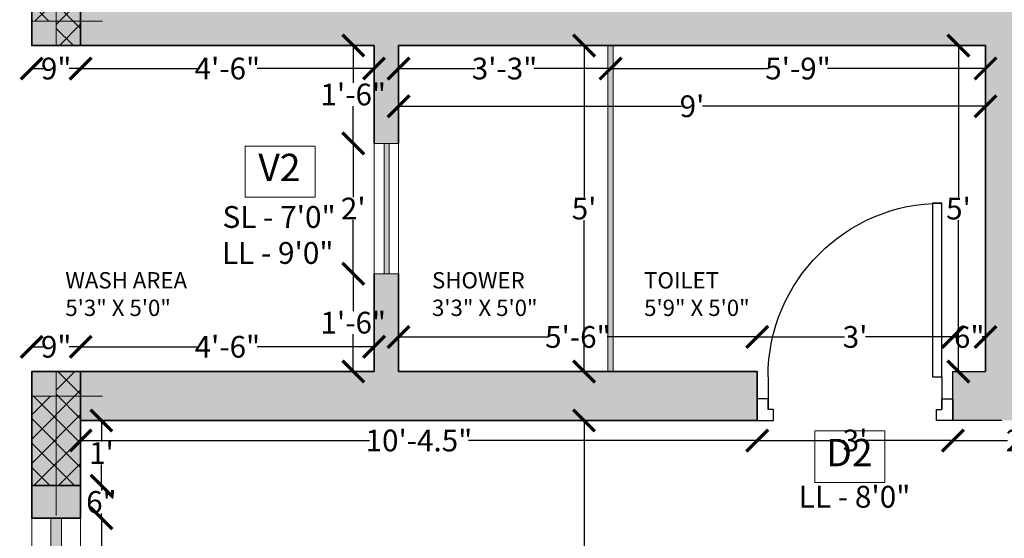
# Model space of a CAD drawing. Units: inches. Extents: x 2 to 905, y 9 to 678.
# Tile 3 of 8: x 114 to 295, y 272 to 367. Entities that reach past the tile are written whole.
import ezdxf

# ---------------------------------------------------------------- set-up
doc = ezdxf.new("R2010")
doc.units = ezdxf.units.IN
doc.linetypes.add('ACAD_ISO02W100', pattern=[15, 12, -3])
for name, color, linetype, lineweight in [('A-ANNO-DIMS', 7, 'Continuous', 18), ('A-COLS', 1, 'Continuous', 35), ('A-COLS-MARK', 1, 'Continuous', 18), ('A-COLS-MARK-PATT', 3, 'Continuous', 13), ('A-COLS-PATT', 1, 'Continuous', 13), ('A-DOOR', 7, 'Continuous', 25), ('A-GLAZ', 4, 'Continuous', 18), ('A-GLAZ-PATT', 4, 'Continuous', 13), ('A-TRAN-HIDN', 7, 'ACAD_ISO02W100', 25), ('A-WALL', 7, 'Continuous', 35), ('A-WALL-HIDN', 7, 'ACAD_ISO02W100', 18)]:
    doc.layers.add(name, color=color, linetype=linetype, lineweight=lineweight)
for name, color, linetype, lineweight, true_color in [('A-ANNO-IDEN', 251, 'Continuous', 18, 0x636466), ('A-AREA-IDEN', 252, 'Continuous', 18, 0x989898), ('A-WALL-PATT', 252, 'Continuous', 13, 0x939598)]:
    doc.layers.add(name, color=color, linetype=linetype, lineweight=lineweight, true_color=true_color)
doc.styles.add('PDF ArialMT', font='arial.ttf')
doc.styles.add('PDF Century Gothic Bold', font='txt')
doc.styles.get("Standard").update_dxf_attribs({"font": 'arial.ttf'})
doc.dimstyles.get("Standard").update_dxf_attribs({"dimtxt": 4, "dimasz": 4, "dimexe": 0.18, "dimexo": 0.0625, "dimgap": 0.09, "dimtad": 0, "dimtih": 1, "dimtoh": 1, "dimdec": 1, "dimzin": 0, "dimdsep": 46, "dimlunit": 3, "dimtxsty": 'Standard', "dimblk": 'ARCHTICK', "dimcen": 0, "dimse1": 1, "dimse2": 1, "dimclrt": 1, "dimadec": 0, "dimazin": 0, "dimtfac": 1, "dimtdec": 1, "dimtofl": 0, "dimtmove": 0, "dimatfit": 3, "dimfxl": 1, "dimtolj": 1, "dimtzin": 0, "dimarcsym": 0})
pattern_1 = [(45, (895.109, 27.1098), (-2.245064, 2.245064), []), (135, (895.109, 27.1098), (-2.245064, -2.245064), [])]

# ---------------------------------------------------------------- blocks, each defined once
blk = doc.blocks.new('*U3')
for p, q in [((0, 0), (0, -6)), ((32, 0), (32, -6))]:
    blk.add_line(p, q)
blk.add_lwpolyline([(0, 0), (0, 32), (1.75, 32), (1.75, 0)], close=True)
blk.add_arc((0, 0), 32, 0, 90)
blk = doc.blocks.new('_ArchTick')
at = {"color": 0, "linetype": 'ByBlock', "const_width": 0.15}
blk.add_lwpolyline([(-0.5, -0.5), (0.5, 0.5)], dxfattribs=at)
blk = doc.blocks.new('*D7')
at = {"layer": 'A-ANNO-DIMS', "color": 0, "lineweight": -2, "transparency": 16777216}
for p, q in [((218.07, 293.58), (218.07, 217.71)), ((218.07, 137.58), (218.07, 213.44))]:
    blk.add_line(p, q, dxfattribs=at)
at = {"layer": 'Defpoints', "color": 0, "transparency": 16777216}
for p in [(218.07, 293.58), (237.93, 293.58), (237.93, 137.58)]:
    blk.add_point(p, dxfattribs=at)
at = {"layer": 'A-ANNO-DIMS', "color": 0, "lineweight": -2, "transparency": 16777216, "xscale": 4, "yscale": 4, "zscale": 4}
for p, rotation in [((218.07, 293.58), 90), ((218.07, 137.58), 270)]:
    blk.add_blockref('_ArchTick', p, dxfattribs=dict(at, rotation=rotation))
at = {"layer": 'A-ANNO-DIMS', "color": 0, "transparency": 16777216, "insert": (218.07, 215.58), "char_height": 4, "attachment_point": 5}
blk.add_mtext("\\A1;13'", dxfattribs=at)
blk = doc.blocks.new('*D9')
at = {"layer": 'A-ANNO-DIMS', "color": 0, "lineweight": -2, "transparency": 16777216}
for p, q in [((218.07, 362.58), (218.07, 334.7)), ((218.07, 302.58), (218.07, 330.45))]:
    blk.add_line(p, q, dxfattribs=at)
at = {"layer": 'Defpoints', "color": 0, "transparency": 16777216}
for p in [(183.93, 362.58), (183.93, 302.58), (218.07, 302.58)]:
    blk.add_point(p, dxfattribs=at)
at = {"layer": 'A-ANNO-DIMS', "color": 0, "lineweight": -2, "transparency": 16777216, "xscale": 4, "yscale": 4, "zscale": 4}
for p, rotation in [((218.07, 362.58), 90), ((218.07, 302.58), 270)]:
    blk.add_blockref('_ArchTick', p, dxfattribs=dict(at, rotation=rotation))
at = {"layer": 'A-ANNO-DIMS', "color": 0, "transparency": 16777216, "insert": (218.07, 332.58), "char_height": 4, "attachment_point": 5}
blk.add_mtext("\\A1;5'", dxfattribs=at)
blk = doc.blocks.new('*D10')
at = {"layer": 'A-ANNO-DIMS', "color": 0, "lineweight": -2, "transparency": 16777216}
for p, q in [((183.93, 351.41), (236, 351.41)), ((291.93, 351.41), (239.86, 351.41))]:
    blk.add_line(p, q, dxfattribs=at)
at = {"layer": 'Defpoints', "color": 0, "transparency": 16777216}
for p in [(183.93, 362.58), (291.93, 362.58), (291.93, 351.41)]:
    blk.add_point(p, dxfattribs=at)
at = {"layer": 'A-ANNO-DIMS', "color": 0, "lineweight": -2, "transparency": 16777216, "xscale": 4, "yscale": 4, "zscale": 4, "rotation": 180}
blk.add_blockref('_ArchTick', (183.93, 351.41), dxfattribs=at)
at = {"layer": 'A-ANNO-DIMS', "color": 0, "lineweight": -2, "transparency": 16777216, "xscale": 4, "yscale": 4, "zscale": 4}
blk.add_blockref('_ArchTick', (291.93, 351.41), dxfattribs=at)
at = {"layer": 'A-ANNO-DIMS', "color": 0, "transparency": 16777216, "insert": (237.93, 351.41), "char_height": 4, "attachment_point": 5}
blk.add_mtext("\\A1;9'", dxfattribs=at)
blk = doc.blocks.new('*D25')
at = {"layer": 'A-ANNO-DIMS', "color": 0, "lineweight": -2, "transparency": 16777216}
for p, q in [((129.26, 275.58), (129.26, 253.67)), ((129.26, 227.58), (129.26, 249.49))]:
    blk.add_line(p, q, dxfattribs=at)
at = {"layer": 'Defpoints', "color": 0, "transparency": 16777216}
for p in [(125.43, 275.58), (129.26, 275.58), (125.43, 227.58)]:
    blk.add_point(p, dxfattribs=at)
at = {"layer": 'A-ANNO-DIMS', "color": 0, "lineweight": -2, "transparency": 16777216, "xscale": 4, "yscale": 4, "zscale": 4}
for p, rotation in [((129.26, 275.58), 90), ((129.26, 227.58), 270)]:
    blk.add_blockref('_ArchTick', p, dxfattribs=dict(at, rotation=rotation))
at = {"layer": 'A-ANNO-DIMS', "color": 0, "transparency": 16777216, "insert": (129.26, 251.58), "char_height": 4, "attachment_point": 5}
blk.add_mtext("\\A1;4'", dxfattribs=at)
blk = doc.blocks.new('*D26')
at = {"layer": 'A-ANNO-DIMS', "color": 0, "lineweight": -2, "transparency": 16777216}
for p, q in [((129.26, 281.58), (129.26, 280.71)), ((129.26, 275.58), (129.26, 276.45))]:
    blk.add_line(p, q, dxfattribs=at)
at = {"layer": 'Defpoints', "color": 0, "transparency": 16777216}
for p in [(125.43, 281.58), (129.26, 281.58), (125.43, 275.58)]:
    blk.add_point(p, dxfattribs=at)
at = {"layer": 'A-ANNO-DIMS', "color": 0, "lineweight": -2, "transparency": 16777216, "xscale": 4, "yscale": 4, "zscale": 4}
for p, rotation in [((129.26, 281.58), 90), ((129.26, 275.58), 270)]:
    blk.add_blockref('_ArchTick', p, dxfattribs=dict(at, rotation=rotation))
at = {"layer": 'A-ANNO-DIMS', "color": 0, "transparency": 16777216, "insert": (129.26, 278.58), "char_height": 4, "attachment_point": 5}
blk.add_mtext('\\A1;6"', dxfattribs=at)
blk = doc.blocks.new('*D27')
at = {"layer": 'A-ANNO-DIMS', "color": 0, "lineweight": -2, "transparency": 16777216}
for p, q in [((129.26, 293.58), (129.26, 289.68)), ((129.26, 281.58), (129.26, 285.48))]:
    blk.add_line(p, q, dxfattribs=at)
at = {"layer": 'Defpoints', "color": 0, "transparency": 16777216}
for p in [(125.43, 293.58), (129.26, 293.58), (125.43, 281.58)]:
    blk.add_point(p, dxfattribs=at)
at = {"layer": 'A-ANNO-DIMS', "color": 0, "lineweight": -2, "transparency": 16777216, "xscale": 4, "yscale": 4, "zscale": 4}
for p, rotation in [((129.26, 293.58), 90), ((129.26, 281.58), 270)]:
    blk.add_blockref('_ArchTick', p, dxfattribs=dict(at, rotation=rotation))
at = {"layer": 'A-ANNO-DIMS', "color": 0, "transparency": 16777216, "insert": (129.26, 287.58), "char_height": 4, "attachment_point": 5}
blk.add_mtext("\\A1;1'", dxfattribs=at)
blk = doc.blocks.new('*D28')
at = {"layer": 'A-ANNO-DIMS', "color": 0, "lineweight": -2, "transparency": 16777216}
for p, q in [((125.43, 289.89), (178.58, 289.89)), ((249.93, 289.89), (196.79, 289.89))]:
    blk.add_line(p, q, dxfattribs=at)
at = {"layer": 'Defpoints', "color": 0, "transparency": 16777216}
for p in [(125.43, 293.58), (249.93, 293.58), (249.93, 289.89)]:
    blk.add_point(p, dxfattribs=at)
at = {"layer": 'A-ANNO-DIMS', "color": 0, "lineweight": -2, "transparency": 16777216, "xscale": 4, "yscale": 4, "zscale": 4, "rotation": 180}
blk.add_blockref('_ArchTick', (125.43, 289.89), dxfattribs=at)
at = {"layer": 'A-ANNO-DIMS', "color": 0, "lineweight": -2, "transparency": 16777216, "xscale": 4, "yscale": 4, "zscale": 4}
blk.add_blockref('_ArchTick', (249.93, 289.89), dxfattribs=at)
at = {"layer": 'A-ANNO-DIMS', "color": 0, "transparency": 16777216, "insert": (187.68, 289.89), "char_height": 4, "attachment_point": 5}
blk.add_mtext('\\A1;10\'-4.5"', dxfattribs=at)
blk = doc.blocks.new('*D29')
at = {"layer": 'A-ANNO-DIMS', "color": 0, "lineweight": -2, "transparency": 16777216}
for p, q in [((249.93, 289.89), (266, 289.89)), ((285.93, 289.89), (269.86, 289.89))]:
    blk.add_line(p, q, dxfattribs=at)
at = {"layer": 'Defpoints', "color": 0, "transparency": 16777216}
for p in [(249.93, 293.58), (285.93, 293.58), (285.93, 289.89)]:
    blk.add_point(p, dxfattribs=at)
at = {"layer": 'A-ANNO-DIMS', "color": 0, "lineweight": -2, "transparency": 16777216, "xscale": 4, "yscale": 4, "zscale": 4, "rotation": 180}
blk.add_blockref('_ArchTick', (249.93, 289.89), dxfattribs=at)
at = {"layer": 'A-ANNO-DIMS', "color": 0, "lineweight": -2, "transparency": 16777216, "xscale": 4, "yscale": 4, "zscale": 4}
blk.add_blockref('_ArchTick', (285.93, 289.89), dxfattribs=at)
at = {"layer": 'A-ANNO-DIMS', "color": 0, "transparency": 16777216, "insert": (267.93, 289.89), "char_height": 4, "attachment_point": 5}
blk.add_mtext("\\A1;3'", dxfattribs=at)
blk = doc.blocks.new('*D30')
at = {"layer": 'A-ANNO-DIMS', "color": 0, "lineweight": -2, "transparency": 16777216}
for p, q in [((285.93, 289.89), (295.97, 289.89)), ((309.93, 289.89), (299.9, 289.89))]:
    blk.add_line(p, q, dxfattribs=at)
at = {"layer": 'Defpoints', "color": 0, "transparency": 16777216}
for p in [(285.93, 293.58), (309.93, 293.58), (309.93, 289.89)]:
    blk.add_point(p, dxfattribs=at)
at = {"layer": 'A-ANNO-DIMS', "color": 0, "lineweight": -2, "transparency": 16777216, "xscale": 4, "yscale": 4, "zscale": 4, "rotation": 180}
blk.add_blockref('_ArchTick', (285.93, 289.89), dxfattribs=at)
at = {"layer": 'A-ANNO-DIMS', "color": 0, "lineweight": -2, "transparency": 16777216, "xscale": 4, "yscale": 4, "zscale": 4}
blk.add_blockref('_ArchTick', (309.93, 289.89), dxfattribs=at)
at = {"layer": 'A-ANNO-DIMS', "color": 0, "transparency": 16777216, "insert": (297.93, 289.89), "char_height": 4, "attachment_point": 5}
blk.add_mtext("\\A1;2'", dxfattribs=at)
blk = doc.blocks.new('*D32')
at = {"layer": 'A-ANNO-DIMS', "color": 0, "lineweight": -2, "transparency": 16777216}
for p, q in [((116.43, 307.14), (118.54, 307.14)), ((125.43, 307.14), (123.32, 307.14))]:
    blk.add_line(p, q, dxfattribs=at)
at = {"layer": 'Defpoints', "color": 0, "transparency": 16777216}
for p in [(125.43, 307.14), (116.43, 302.58), (125.43, 302.58)]:
    blk.add_point(p, dxfattribs=at)
at = {"layer": 'A-ANNO-DIMS', "color": 0, "lineweight": -2, "transparency": 16777216, "xscale": 4, "yscale": 4, "zscale": 4, "rotation": 180}
blk.add_blockref('_ArchTick', (116.43, 307.14), dxfattribs=at)
at = {"layer": 'A-ANNO-DIMS', "color": 0, "lineweight": -2, "transparency": 16777216, "xscale": 4, "yscale": 4, "zscale": 4}
blk.add_blockref('_ArchTick', (125.43, 307.14), dxfattribs=at)
at = {"layer": 'A-ANNO-DIMS', "color": 0, "transparency": 16777216, "insert": (120.93, 307.14), "char_height": 4, "attachment_point": 5}
blk.add_mtext('\\A1;9"', dxfattribs=at)
blk = doc.blocks.new('*D33')
at = {"layer": 'A-ANNO-DIMS', "color": 0, "lineweight": -2, "transparency": 16777216}
for p, q in [((125.43, 307.14), (146.95, 307.14)), ((179.43, 307.14), (157.92, 307.14))]:
    blk.add_line(p, q, dxfattribs=at)
at = {"layer": 'Defpoints', "color": 0, "transparency": 16777216}
for p in [(179.43, 307.14), (125.43, 302.58), (179.43, 302.58)]:
    blk.add_point(p, dxfattribs=at)
at = {"layer": 'A-ANNO-DIMS', "color": 0, "lineweight": -2, "transparency": 16777216, "xscale": 4, "yscale": 4, "zscale": 4, "rotation": 180}
blk.add_blockref('_ArchTick', (125.43, 307.14), dxfattribs=at)
at = {"layer": 'A-ANNO-DIMS', "color": 0, "lineweight": -2, "transparency": 16777216, "xscale": 4, "yscale": 4, "zscale": 4}
blk.add_blockref('_ArchTick', (179.43, 307.14), dxfattribs=at)
at = {"layer": 'A-ANNO-DIMS', "color": 0, "transparency": 16777216, "insert": (152.43, 307.14), "char_height": 4, "attachment_point": 5}
blk.add_mtext('\\A1;4\'-6"', dxfattribs=at)
blk = doc.blocks.new('*D34')
at = {"layer": 'A-ANNO-DIMS', "color": 0, "lineweight": -2, "transparency": 16777216}
for p, q in [((116.43, 358.35), (118.54, 358.35)), ((125.43, 358.35), (123.32, 358.35))]:
    blk.add_line(p, q, dxfattribs=at)
at = {"layer": 'Defpoints', "color": 0, "transparency": 16777216}
for p in [(116.43, 362.58), (125.43, 362.58), (125.43, 358.35)]:
    blk.add_point(p, dxfattribs=at)
at = {"layer": 'A-ANNO-DIMS', "color": 0, "lineweight": -2, "transparency": 16777216, "xscale": 4, "yscale": 4, "zscale": 4, "rotation": 180}
blk.add_blockref('_ArchTick', (116.43, 358.35), dxfattribs=at)
at = {"layer": 'A-ANNO-DIMS', "color": 0, "lineweight": -2, "transparency": 16777216, "xscale": 4, "yscale": 4, "zscale": 4}
blk.add_blockref('_ArchTick', (125.43, 358.35), dxfattribs=at)
at = {"layer": 'A-ANNO-DIMS', "color": 0, "transparency": 16777216, "insert": (120.93, 358.35), "char_height": 4, "attachment_point": 5}
blk.add_mtext('\\A1;9"', dxfattribs=at)
blk = doc.blocks.new('*D35')
at = {"layer": 'A-ANNO-DIMS', "color": 0, "lineweight": -2, "transparency": 16777216}
for p, q in [((125.43, 358.35), (146.95, 358.35)), ((179.43, 358.35), (157.92, 358.35))]:
    blk.add_line(p, q, dxfattribs=at)
at = {"layer": 'Defpoints', "color": 0, "transparency": 16777216}
for p in [(125.43, 362.58), (179.43, 362.58), (179.43, 358.35)]:
    blk.add_point(p, dxfattribs=at)
at = {"layer": 'A-ANNO-DIMS', "color": 0, "lineweight": -2, "transparency": 16777216, "xscale": 4, "yscale": 4, "zscale": 4, "rotation": 180}
blk.add_blockref('_ArchTick', (125.43, 358.35), dxfattribs=at)
at = {"layer": 'A-ANNO-DIMS', "color": 0, "lineweight": -2, "transparency": 16777216, "xscale": 4, "yscale": 4, "zscale": 4}
blk.add_blockref('_ArchTick', (179.43, 358.35), dxfattribs=at)
at = {"layer": 'A-ANNO-DIMS', "color": 0, "transparency": 16777216, "insert": (152.43, 358.35), "char_height": 4, "attachment_point": 5}
blk.add_mtext('\\A1;4\'-6"', dxfattribs=at)
blk = doc.blocks.new('*D36')
at = {"layer": 'A-ANNO-DIMS', "color": 0, "lineweight": -2, "transparency": 16777216}
for p, q in [((175.6, 320.58), (175.6, 313.71)), ((175.6, 302.58), (175.6, 309.45))]:
    blk.add_line(p, q, dxfattribs=at)
at = {"layer": 'Defpoints', "color": 0, "transparency": 16777216}
for p in [(175.6, 320.58), (179.43, 320.58), (179.43, 302.58)]:
    blk.add_point(p, dxfattribs=at)
at = {"layer": 'A-ANNO-DIMS', "color": 0, "lineweight": -2, "transparency": 16777216, "xscale": 4, "yscale": 4, "zscale": 4}
for p, rotation in [((175.6, 320.58), 90), ((175.6, 302.58), 270)]:
    blk.add_blockref('_ArchTick', p, dxfattribs=dict(at, rotation=rotation))
at = {"layer": 'A-ANNO-DIMS', "color": 0, "transparency": 16777216, "insert": (175.6, 311.58), "char_height": 4, "attachment_point": 5}
blk.add_mtext('\\A1;1\'-6"', dxfattribs=at)
blk = doc.blocks.new('*D37')
at = {"layer": 'A-ANNO-DIMS', "color": 0, "lineweight": -2, "transparency": 16777216}
for p, q in [((175.6, 344.58), (175.6, 334.68)), ((175.6, 320.58), (175.6, 330.48))]:
    blk.add_line(p, q, dxfattribs=at)
at = {"layer": 'Defpoints', "color": 0, "transparency": 16777216}
for p in [(175.6, 344.58), (179.43, 344.58), (179.43, 320.58)]:
    blk.add_point(p, dxfattribs=at)
at = {"layer": 'A-ANNO-DIMS', "color": 0, "lineweight": -2, "transparency": 16777216, "xscale": 4, "yscale": 4, "zscale": 4}
for p, rotation in [((175.6, 344.58), 90), ((175.6, 320.58), 270)]:
    blk.add_blockref('_ArchTick', p, dxfattribs=dict(at, rotation=rotation))
at = {"layer": 'A-ANNO-DIMS', "color": 0, "transparency": 16777216, "insert": (175.6, 332.58), "char_height": 4, "attachment_point": 5}
blk.add_mtext("\\A1;2'", dxfattribs=at)
blk = doc.blocks.new('*D38')
at = {"layer": 'A-ANNO-DIMS', "color": 0, "lineweight": -2, "transparency": 16777216}
for p, q in [((175.6, 362.58), (175.6, 355.71)), ((175.6, 344.58), (175.6, 351.45))]:
    blk.add_line(p, q, dxfattribs=at)
at = {"layer": 'Defpoints', "color": 0, "transparency": 16777216}
for p in [(175.6, 362.58), (179.43, 362.58), (179.43, 344.58)]:
    blk.add_point(p, dxfattribs=at)
at = {"layer": 'A-ANNO-DIMS', "color": 0, "lineweight": -2, "transparency": 16777216, "xscale": 4, "yscale": 4, "zscale": 4}
for p, rotation in [((175.6, 362.58), 90), ((175.6, 344.58), 270)]:
    blk.add_blockref('_ArchTick', p, dxfattribs=dict(at, rotation=rotation))
at = {"layer": 'A-ANNO-DIMS', "color": 0, "transparency": 16777216, "insert": (175.6, 353.58), "char_height": 4, "attachment_point": 5}
blk.add_mtext('\\A1;1\'-6"', dxfattribs=at)
blk = doc.blocks.new('*D39')
at = {"layer": 'A-ANNO-DIMS', "color": 0, "lineweight": -2, "transparency": 16777216}
for p, q in [((183.93, 358.35), (198.03, 358.35)), ((222.93, 358.35), (208.84, 358.35))]:
    blk.add_line(p, q, dxfattribs=at)
at = {"layer": 'Defpoints', "color": 0, "transparency": 16777216}
for p in [(183.93, 362.58), (222.93, 362.58), (222.93, 358.35)]:
    blk.add_point(p, dxfattribs=at)
at = {"layer": 'A-ANNO-DIMS', "color": 0, "lineweight": -2, "transparency": 16777216, "xscale": 4, "yscale": 4, "zscale": 4, "rotation": 180}
blk.add_blockref('_ArchTick', (183.93, 358.35), dxfattribs=at)
at = {"layer": 'A-ANNO-DIMS', "color": 0, "lineweight": -2, "transparency": 16777216, "xscale": 4, "yscale": 4, "zscale": 4}
blk.add_blockref('_ArchTick', (222.93, 358.35), dxfattribs=at)
at = {"layer": 'A-ANNO-DIMS', "color": 0, "transparency": 16777216, "insert": (203.43, 358.35), "char_height": 4, "attachment_point": 5}
blk.add_mtext('\\A1;3\'-3"', dxfattribs=at)
blk = doc.blocks.new('*D40')
at = {"layer": 'A-ANNO-DIMS', "color": 0, "lineweight": -2, "transparency": 16777216}
for p, q in [((222.93, 358.35), (252.03, 358.35)), ((291.93, 358.35), (262.84, 358.35))]:
    blk.add_line(p, q, dxfattribs=at)
at = {"layer": 'Defpoints', "color": 0, "transparency": 16777216}
for p in [(222.93, 362.58), (291.93, 362.58), (291.93, 358.35)]:
    blk.add_point(p, dxfattribs=at)
at = {"layer": 'A-ANNO-DIMS', "color": 0, "lineweight": -2, "transparency": 16777216, "xscale": 4, "yscale": 4, "zscale": 4, "rotation": 180}
blk.add_blockref('_ArchTick', (222.93, 358.35), dxfattribs=at)
at = {"layer": 'A-ANNO-DIMS', "color": 0, "lineweight": -2, "transparency": 16777216, "xscale": 4, "yscale": 4, "zscale": 4}
blk.add_blockref('_ArchTick', (291.93, 358.35), dxfattribs=at)
at = {"layer": 'A-ANNO-DIMS', "color": 0, "transparency": 16777216, "insert": (257.43, 358.35), "char_height": 4, "attachment_point": 5}
blk.add_mtext('\\A1;5\'-9"', dxfattribs=at)
blk = doc.blocks.new('*D44')
at = {"layer": 'A-ANNO-DIMS', "color": 0, "lineweight": -2, "transparency": 16777216}
for p, q in [((183.93, 308.95), (211.53, 308.95)), ((249.93, 308.95), (222.34, 308.95))]:
    blk.add_line(p, q, dxfattribs=at)
at = {"layer": 'Defpoints', "color": 0, "transparency": 16777216}
for p in [(249.93, 308.95), (183.93, 302.58), (249.93, 302.58)]:
    blk.add_point(p, dxfattribs=at)
at = {"layer": 'A-ANNO-DIMS', "color": 0, "lineweight": -2, "transparency": 16777216, "xscale": 4, "yscale": 4, "zscale": 4, "rotation": 180}
blk.add_blockref('_ArchTick', (183.93, 308.95), dxfattribs=at)
at = {"layer": 'A-ANNO-DIMS', "color": 0, "lineweight": -2, "transparency": 16777216, "xscale": 4, "yscale": 4, "zscale": 4}
blk.add_blockref('_ArchTick', (249.93, 308.95), dxfattribs=at)
at = {"layer": 'A-ANNO-DIMS', "color": 0, "transparency": 16777216, "insert": (216.93, 308.95), "char_height": 4, "attachment_point": 5}
blk.add_mtext('\\A1;5\'-6"', dxfattribs=at)
blk = doc.blocks.new('*D45')
at = {"layer": 'A-ANNO-DIMS', "color": 0, "lineweight": -2, "transparency": 16777216}
for p, q in [((249.93, 308.95), (266, 308.95)), ((285.93, 308.95), (269.86, 308.95))]:
    blk.add_line(p, q, dxfattribs=at)
at = {"layer": 'Defpoints', "color": 0, "transparency": 16777216}
for p in [(285.93, 308.95), (249.93, 302.58), (285.93, 302.58)]:
    blk.add_point(p, dxfattribs=at)
at = {"layer": 'A-ANNO-DIMS', "color": 0, "lineweight": -2, "transparency": 16777216, "xscale": 4, "yscale": 4, "zscale": 4, "rotation": 180}
blk.add_blockref('_ArchTick', (249.93, 308.95), dxfattribs=at)
at = {"layer": 'A-ANNO-DIMS', "color": 0, "lineweight": -2, "transparency": 16777216, "xscale": 4, "yscale": 4, "zscale": 4}
blk.add_blockref('_ArchTick', (285.93, 308.95), dxfattribs=at)
at = {"layer": 'A-ANNO-DIMS', "color": 0, "transparency": 16777216, "insert": (267.93, 308.95), "char_height": 4, "attachment_point": 5}
blk.add_mtext("\\A1;3'", dxfattribs=at)
blk = doc.blocks.new('*D46')
at = {"layer": 'A-ANNO-DIMS', "color": 0, "lineweight": -2, "transparency": 16777216}
for p, q in [((285.93, 308.95), (286.53, 308.95)), ((291.93, 308.95), (291.33, 308.95))]:
    blk.add_line(p, q, dxfattribs=at)
at = {"layer": 'Defpoints', "color": 0, "transparency": 16777216}
for p in [(291.93, 308.95), (285.93, 302.58), (291.93, 302.58)]:
    blk.add_point(p, dxfattribs=at)
at = {"layer": 'A-ANNO-DIMS', "color": 0, "lineweight": -2, "transparency": 16777216, "xscale": 4, "yscale": 4, "zscale": 4, "rotation": 180}
blk.add_blockref('_ArchTick', (285.93, 308.95), dxfattribs=at)
at = {"layer": 'A-ANNO-DIMS', "color": 0, "lineweight": -2, "transparency": 16777216, "xscale": 4, "yscale": 4, "zscale": 4}
blk.add_blockref('_ArchTick', (291.93, 308.95), dxfattribs=at)
at = {"layer": 'A-ANNO-DIMS', "color": 0, "transparency": 16777216, "insert": (288.93, 308.95), "char_height": 4, "attachment_point": 5}
blk.add_mtext('\\A1;6"', dxfattribs=at)
blk = doc.blocks.new('*D47')
at = {"layer": 'A-ANNO-DIMS', "color": 0, "lineweight": -2, "transparency": 16777216}
for p, q in [((286.96, 362.58), (286.96, 334.7)), ((286.96, 302.58), (286.96, 330.45))]:
    blk.add_line(p, q, dxfattribs=at)
at = {"layer": 'Defpoints', "color": 0, "transparency": 16777216}
for p in [(291.93, 362.58), (286.96, 302.58), (291.93, 302.58)]:
    blk.add_point(p, dxfattribs=at)
at = {"layer": 'A-ANNO-DIMS', "color": 0, "lineweight": -2, "transparency": 16777216, "xscale": 4, "yscale": 4, "zscale": 4}
for p, rotation in [((286.96, 362.58), 90), ((286.96, 302.58), 270)]:
    blk.add_blockref('_ArchTick', p, dxfattribs=dict(at, rotation=rotation))
at = {"layer": 'A-ANNO-DIMS', "color": 0, "transparency": 16777216, "insert": (286.96, 332.58), "char_height": 4, "attachment_point": 5}
blk.add_mtext("\\A1;5'", dxfattribs=at)
blk = doc.blocks.new('COL-DATUM-L')
h = blk.add_hatch(color=256)
h.dxf.hatch_style = 1
h.paths.add_polyline_path([(4.5, 0), (4.5, 4.5), (0, 4.5), (0, 0)])
for p, q in [((4.5, 0), (4.5, 26.48)), ((0, 4.5), (13.01, 4.5))]:
    blk.add_line(p, q)
blk.add_lwpolyline([(4.5, 0), (0, 0), (0, 4.5), (4.5, 4.5)], close=True)
blk = doc.blocks.new('GLAZ-W4-48')
h = blk.add_hatch(color=256)
h.dxf.hatch_style = 1
h.paths.add_polyline_path([(48, 0), (48, 2), (0, 2), (0, 0)])
for p, q in [((0, 2), (48, 2)), ((0, 0), (48, 0))]:
    blk.add_line(p, q)
blk = doc.blocks.new('GLAZ-V2-24')
h = blk.add_hatch(color=256)
h.dxf.hatch_style = 1
h.paths.add_polyline_path([(0.97, 24), (0, 24), (0, 0), (0.97, 0)])
for p, q in [((0, 0), (0, 24)), ((0.97, 0), (0.97, 24))]:
    blk.add_line(p, q)

msp = doc.modelspace()

# ---------------------------------------------------------------- hatches: boundary and pattern name
at = {"layer": 'A-COLS-MARK-PATT'}
h = msp.add_hatch(color=256, dxfattribs=at)
h.dxf.hatch_style = 1
h.paths.add_polyline_path([(116.43, 302.58), (116.43, 298.08), (120.93, 298.08), (120.93, 302.58)])
at = {"layer": 'A-COLS-PATT'}
h = msp.add_hatch(dxfattribs=at)
h.set_pattern_fill('ANSI37', color=256)
h.set_pattern_definition(pattern_1)
h.paths.add_polyline_path([(125.43, 367.08), (120.93, 367.08), (120.93, 362.58), (125.43, 362.58)])
h.paths.add_polyline_path([(125.43, 383.58), (120.93, 383.58), (120.93, 367.08), (125.43, 367.08)])
h.paths.add_polyline_path([(120.93, 383.58), (116.43, 383.58), (116.43, 367.08), (120.93, 367.08)])
h = msp.add_hatch(dxfattribs=at)
h.set_pattern_fill('ANSI37', color=256)
h.set_pattern_definition(pattern_1)
h.paths.add_polyline_path([(125.43, 298.08), (120.93, 298.08), (120.93, 302.58), (125.43, 302.58)])
h.paths.add_polyline_path([(125.43, 281.58), (120.93, 281.58), (120.93, 298.08), (125.43, 298.08)])
h.paths.add_polyline_path([(120.93, 281.58), (116.43, 281.58), (116.43, 298.08), (120.93, 298.08)])
at = {"layer": 'A-GLAZ-PATT'}
h = msp.add_hatch(color=256, dxfattribs=at)
h.dxf.hatch_style = 1
h.paths.add_polyline_path([(223.43, 362.58), (222.43, 362.58), (222.43, 302.58), (223.43, 302.58)])
at = {"layer": 'A-WALL-PATT'}
h = msp.add_hatch(color=256, dxfattribs=at)
h.dxf.hatch_style = 1
h.paths.add_polyline_path([(125.43, 227.58), (116.43, 227.58), (116.43, 128.58), (237.93, 128.58), (237.93, 137.58), (125.43, 137.58)])
h.paths.add_polyline_path([(249.93, 302.58), (183.93, 302.58), (183.93, 320.58), (179.43, 320.58), (179.43, 302.58), (116.43, 302.58), (116.43, 275.58), (125.43, 275.58), (125.43, 293.58), (249.93, 293.58), (249.93, 297.58)], flags=0)
h.paths.add_polyline_path([(369.93, 137.58), (360.93, 137.58), (360.93, 218.58), (369.93, 218.58), (369.93, 227.58), (363.93, 227.58), (351.93, 227.58), (351.93, 137.58), (345.93, 137.58), (345.93, 128.58), (360.93, 128.58), (369.93, 128.58)])
h.paths.add_polyline_path([(297.93, 137.58), (285.93, 137.58), (285.93, 128.58), (297.93, 128.58)])
h.paths.add_polyline_path([(369.93, 444.58), (360.93, 444.58), (360.93, 371.58), (183.93, 371.58), (183.93, 460.08), (125.43, 460.08), (125.43, 466.08), (116.43, 466.08), (116.43, 449.58), (120.43, 449.58), (125.43, 449.58), (125.43, 455.58), (179.43, 455.58), (179.43, 371.58), (125.43, 371.58), (125.43, 389.58), (116.43, 389.58), (116.43, 362.58), (179.43, 362.58), (179.43, 344.58), (183.93, 344.58), (183.93, 362.58), (291.93, 362.58), (291.93, 302.58), (285.93, 302.58), (285.93, 293.58), (309.93, 293.58), (309.93, 302.58), (300.93, 302.58), (300.93, 362.58), (360.93, 362.58), (360.93, 302.58), (351.93, 302.58), (351.93, 293.58), (360.93, 293.58), (360.93, 275.58), (363.93, 275.58), (369.93, 275.58)])
h.paths.add_polyline_path([(282.93, 557.58), (116.43, 557.58), (116.43, 506.08), (120.43, 506.08), (125.43, 506.08), (125.43, 548.58), (282.93, 548.58)])
h.paths.add_polyline_path([(369.93, 557.58), (330.93, 557.58), (330.93, 548.58), (360.93, 548.58), (360.93, 504.58), (369.93, 504.58)])
h = msp.add_hatch(color=256, dxfattribs=at)
h.dxf.hatch_style = 1
h.paths.add_polyline_path([(116.43, 302.58), (116.43, 275.58), (125.43, 275.58), (125.43, 293.58), (249.93, 293.58), (249.93, 297.58), (249.93, 302.58), (183.93, 302.58), (183.93, 320.58), (179.43, 320.58), (179.43, 302.58)])

# ---------------------------------------------------------------- linework, layer by layer
at = {"layer": 'A-ANNO-IDEN'}
for points in [[(155.7, 344.04), (168.6, 344.04), (168.6, 334.67), (155.7, 334.67)], [(260.53, 291.67), (273.43, 291.67), (273.43, 282.19), (260.53, 282.19)]]:
    msp.add_lwpolyline(points, close=True, dxfattribs=at)
at = {"layer": 'A-COLS'}
for points in [[(116.43, 383.58), (125.43, 383.58), (125.43, 362.58), (116.43, 362.58)], [(116.43, 281.58), (125.43, 281.58), (125.43, 302.58), (116.43, 302.58)]]:
    msp.add_lwpolyline(points, close=True, dxfattribs=at)
at = {"layer": 'A-COLS-MARK'}
for p, q in [((120.93, 302.58), (120.93, 276.1)), ((116.43, 298.08), (129.44, 298.08))]:
    msp.add_line(p, q, dxfattribs=at)
msp.add_lwpolyline([(120.93, 302.58), (116.43, 302.58), (116.43, 298.08), (120.93, 298.08)], close=True, dxfattribs=at)
at = {"layer": 'A-DOOR'}
for points in [[(252.93, 293.58), (252.93, 295.58), (251.93, 295.58), (251.93, 297.58), (249.93, 297.58), (249.93, 293.58)], [(282.93, 293.58), (282.93, 295.58), (283.93, 295.58), (283.93, 297.58), (285.93, 297.58), (285.93, 293.58)]]:
    msp.add_lwpolyline(points, close=True, dxfattribs=at)
at = {"layer": 'A-GLAZ'}
for p, q in [((222.43, 362.58), (222.43, 302.58)), ((223.43, 362.58), (223.43, 302.58))]:
    msp.add_line(p, q, dxfattribs=at)
for points in [[(179.43, 320.58), (179.43, 344.58), (183.93, 344.58), (183.93, 320.58)], [(116.43, 227.58), (116.43, 275.58), (125.43, 275.58), (125.43, 227.58)]]:
    msp.add_lwpolyline(points, close=True, dxfattribs=at)
at = {"layer": 'A-TRAN-HIDN'}
msp.add_lwpolyline([(360.93, 302.58), (360.93, 362.58), (300.93, 362.58), (300.93, 302.58), (309.93, 302.58), (351.93, 302.58), (309.93, 293.58), (351.93, 293.58), (309.93, 302.58), (309.93, 293.58), (285.93, 293.58), (285.93, 302.58), (291.93, 302.58)], dxfattribs=at)
at = {"layer": 'A-WALL'}
for p, q in [((116.43, 389.58), (116.43, 362.58)), ((116.43, 362.58), (179.43, 362.58)), ((179.43, 362.58), (179.43, 344.58)), ((183.93, 362.58), (183.93, 344.58)), ((183.93, 362.58), (291.93, 362.58)), ((291.93, 362.58), (291.93, 302.58)), ((179.43, 320.58), (179.43, 302.58)), ((183.93, 320.58), (183.93, 302.58)), ((116.43, 302.58), (179.43, 302.58)), ((116.43, 302.58), (116.43, 275.58)), ((183.93, 302.58), (249.93, 302.58)), ((249.93, 293.58), (249.93, 302.58)), ((125.43, 293.58), (249.93, 293.58)), ((125.43, 293.58), (125.43, 275.58)), ((125.43, 275.58), (116.43, 275.58)), ((116.43, 275.58), (125.43, 275.58))]:
    msp.add_line(p, q, dxfattribs=at)
at = {"layer": 'A-WALL-HIDN'}
for p, q in [((179.43, 344.58), (183.93, 344.58)), ((179.43, 320.58), (183.93, 320.58))]:
    msp.add_line(p, q, dxfattribs=at)

# ---------------------------------------------------------------- block references
at = {"layer": 'A-COLS-MARK'}
msp.add_blockref('COL-DATUM-L', (116.43, 362.58), dxfattribs=at)
at = {"layer": 'A-DOOR', "xscale": -1}
msp.add_blockref('*U3', (283.93, 301.58), dxfattribs=at)
at = {"layer": 'A-GLAZ'}
msp.add_blockref('GLAZ-V2-24', (181.26, 320.58), dxfattribs=at)
at = {"layer": 'A-GLAZ', "rotation": 90.00000000000003}
msp.add_blockref('GLAZ-W4-48', (121.93, 227.58), dxfattribs=at)

# ---------------------------------------------------------------- texts
at = {"layer": 'A-ANNO-IDEN', "attachment_point": 4, "style": 'PDF ArialMT'}
for s, insert, char_height in [('V2', (158.14, 339.49), 5.029), ('SL - 7\'0"', (151.53, 330.51), 4.023), ('LL - 9\'0"', (151.42, 323.89), 4.023), ('D2', (262.64, 287.01), 5.029), ('LL - 8\'0"', (257.57, 279.02), 4.023)]:
    msp.add_mtext(s, dxfattribs=dict(at, insert=insert, char_height=char_height))
at = {"layer": 'A-AREA-IDEN', "char_height": 3, "attachment_point": 4, "style": 'PDF Century Gothic Bold'}
for s, insert in [('WASH AREA', (122.62, 318.99)), ('SHOWER', (190.09, 318.99)), ('TOILET', (229.12, 318.99)), ('5\'3" X 5\'0"', (122.62, 313.92)), ('3\'3" X 5\'0"', (190.09, 313.92)), ('5\'9" X 5\'0"', (229.12, 313.92))]:
    msp.add_mtext(s, dxfattribs=dict(at, insert=insert))

# ---------------------------------------------------------------- dimensions: what is measured, and where the dimension line sits
at = {"layer": 'A-ANNO-DIMS'}
for base, p1, p2, override, picture, middle in [((175.6, 362.58), (179.43, 344.58), (179.43, 362.58), {"dimdec": 0, "dimclrd": 0, "dimclre": 0, "dimclrt": 0, "dimtmove": 1}, '*D38', (175.6, 353.58)), ((218.07, 302.58), (183.93, 362.58), (183.93, 302.58), {"dimclrd": 0, "dimclre": 0, "dimclrt": 0}, '*D9', (218.07, 332.58)), ((286.96, 302.58), (291.93, 362.58), (291.93, 302.58), {"dimclrd": 0, "dimclre": 0, "dimclrt": 0}, '*D47', (286.96, 332.58)), ((175.6, 344.58), (179.43, 320.58), (179.43, 344.58), {"dimclrd": 0, "dimclre": 0, "dimclrt": 0, "dimtmove": 1}, '*D37', (175.6, 332.58)), ((175.6, 320.58), (179.43, 302.58), (179.43, 320.58), {"dimdec": 0, "dimclrd": 0, "dimclre": 0, "dimclrt": 0}, '*D36', (175.6, 311.58)), ((129.26, 293.58), (125.43, 281.58), (125.43, 293.58), {"dimclrd": 0, "dimclre": 0, "dimclrt": 0, "dimtmove": 1}, '*D27', (129.26, 287.58)), ((218.07, 293.58), (237.93, 137.58), (237.93, 293.58), {"dimclrd": 0, "dimclre": 0, "dimclrt": 0}, '*D7', (218.07, 215.58)), ((129.26, 281.58), (125.43, 275.58), (125.43, 281.58), {"dimdec": 0, "dimclrd": 0, "dimclre": 0, "dimclrt": 0, "dimtmove": 1}, '*D26', (129.26, 278.58)), ((129.26, 275.58), (125.43, 227.58), (125.43, 275.58), {"dimclrd": 0, "dimclre": 0, "dimclrt": 0, "dimtmove": 1}, '*D25', (129.26, 251.58))]:
    dim = msp.add_linear_dim(base=base, p1=p1, p2=p2, angle=90, dimstyle='Standard', override=override, dxfattribs=at)
    dim.commit()
    dim.dimension.update_dxf_attribs({"geometry": picture, "text_midpoint": middle})
for base, p1, p2, override, picture, middle in [((125.43, 358.35), (116.43, 362.58), (125.43, 362.58), {"dimdec": 0, "dimclrd": 0, "dimclre": 0, "dimclrt": 0}, '*D34', (120.93, 358.35)), ((179.43, 358.35), (125.43, 362.58), (179.43, 362.58), {"dimdec": 0, "dimclrd": 0, "dimclre": 0, "dimclrt": 0}, '*D35', (152.43, 358.35)), ((291.93, 351.41), (183.93, 362.58), (291.93, 362.58), {"dimclrd": 0, "dimclre": 0, "dimclrt": 0}, '*D10', (237.93, 351.41)), ((222.93, 358.35), (183.93, 362.58), (222.93, 362.58), {"dimdec": 0, "dimclrd": 0, "dimclre": 0, "dimclrt": 0}, '*D39', (203.43, 358.35)), ((291.93, 358.35), (222.93, 362.58), (291.93, 362.58), {"dimdec": 0, "dimclrd": 0, "dimclre": 0, "dimclrt": 0, "dimtmove": 1}, '*D40', (257.43, 358.35)), ((249.93, 308.95), (183.93, 302.58), (249.93, 302.58), {"dimdec": 0, "dimclrd": 0, "dimclre": 0, "dimclrt": 0}, '*D44', (216.93, 308.95)), ((285.93, 308.95), (249.93, 302.58), (285.93, 302.58), {"dimclrd": 0, "dimclre": 0, "dimclrt": 0, "dimtmove": 1}, '*D45', (267.93, 308.95)), ((291.93, 308.95), (285.93, 302.58), (291.93, 302.58), {"dimdec": 0, "dimclrd": 0, "dimclre": 0, "dimclrt": 0, "dimtmove": 1}, '*D46', (288.93, 308.95)), ((125.43, 307.14), (116.43, 302.58), (125.43, 302.58), {"dimdec": 0, "dimclrd": 0, "dimclre": 0, "dimclrt": 0}, '*D32', (120.93, 307.14)), ((179.43, 307.14), (125.43, 302.58), (179.43, 302.58), {"dimdec": 0, "dimclrd": 0, "dimclre": 0, "dimclrt": 0}, '*D33', (152.43, 307.14)), ((249.93, 289.89), (125.43, 293.58), (249.93, 293.58), {"dimclrd": 0, "dimclre": 0, "dimclrt": 0}, '*D28', (187.68, 289.89)), ((285.93, 289.89), (249.93, 293.58), (285.93, 293.58), {"dimclrd": 0, "dimclre": 0, "dimclrt": 0, "dimtmove": 1}, '*D29', (267.93, 289.89)), ((309.93, 289.89), (285.93, 293.58), (309.93, 293.58), {"dimclrd": 0, "dimclre": 0, "dimclrt": 0, "dimtmove": 1}, '*D30', (297.93, 289.89))]:
    dim = msp.add_linear_dim(base=base, p1=p1, p2=p2, dimstyle='Standard', override=override, dxfattribs=at)
    dim.commit()
    dim.dimension.update_dxf_attribs({"geometry": picture, "text_midpoint": middle})

doc.saveas('drawing.dxf')
